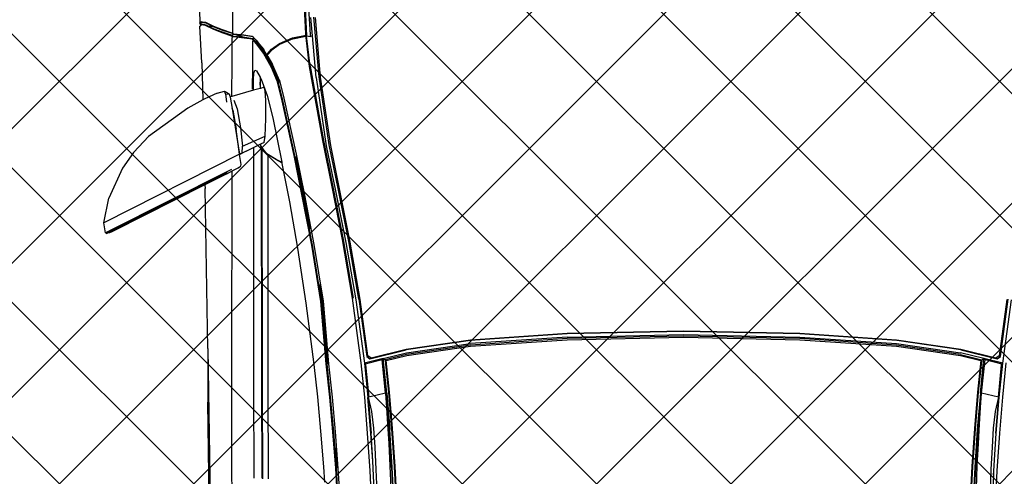
# Model space of a CAD drawing. Units: inches. Extents: x 2167 to 2589, y 1680 to 2489.
# Tile 17 of 38: x 2335 to 2387, y 1772 to 1796. Entities that reach past the tile are written whole.
import ezdxf

# ---------------------------------------------------------------- set-up
doc = ezdxf.new("R2010")
doc.units = ezdxf.units.IN
doc.header["$MEASUREMENT"] = 0
doc.layers.get('0').update_dxf_attribs({"color": 250})
doc.layers.add('C-PRKG-VEHS', color=8, linetype='Continuous', lineweight=13)
doc.layers.add('L-PVMT-PATT', color=252, linetype='Continuous', lineweight=13)
doc.layers.add('Edges', color=250, linetype='Continuous')

# ---------------------------------------------------------------- blocks, each defined once
blk = doc.blocks.new('Nissan Qashqai pl')
at = {"layer": 'Edges'}
for p, q in [((9.2789, 12.5131), (9.1617, 12.5292)), ((9.2669, 12.5088), (9.1605, 12.5233)), ((9.1612, 12.5208), (9.2656, 12.5065)), ((9.2656, 12.5065), (9.2669, 12.5088)), ((9.2707, 12.5028), (9.2669, 12.5088)), ((9.2789, 12.5131), (9.2704, 12.4783)), ((9.2724, 12.4804), (9.2799, 12.5114)), ((9.2783, 12.5191), (9.3422, 12.5126)), ((9.2799, 12.5114), (9.2789, 12.5131)), ((9.3427, 12.5066), (9.2789, 12.5131)), ((9.2819, 12.5112), (9.2799, 12.5114)), ((9.2803, 12.5116), (9.2822, 12.5118)), ((9.3418, 12.5051), (9.2819, 12.5112)), ((9.3422, 12.5126), (9.4088, 12.507)), ((9.2694, 12.5006), (9.2535, 12.4354)), ((9.2543, 12.4356), (9.2707, 12.5028)), ((9.2656, 12.5065), (9.2694, 12.5006)), ((9.2707, 12.5028), (9.2694, 12.5006)), ((9.3418, 12.5051), (9.3346, 12.4741)), ((9.342, 12.5059), (9.3418, 12.5051)), ((9.3687, 12.5), (9.342, 12.5059)), ((9.4087, 12.5003), (9.342, 12.5059)), ((9.4093, 12.5011), (9.3427, 12.5066)), ((9.3992, 12.496), (9.3687, 12.5)), ((9.4347, 12.494), (9.3992, 12.496)), ((9.4087, 12.5003), (9.4688, 12.4968)), ((9.4088, 12.507), (9.4782, 12.5024)), ((9.4785, 12.4965), (9.4093, 12.5011)), ((9.4761, 12.4919), (9.4347, 12.494)), ((9.4688, 12.4968), (9.4789, 12.4964)), ((9.5168, 12.4903), (9.4761, 12.4919)), ((9.4782, 12.5024), (9.5503, 12.4987)), ((9.4789, 12.4964), (9.4785, 12.4965)), ((9.4862, 12.4961), (9.4785, 12.4965)), ((9.4789, 12.4964), (9.4862, 12.4961)), ((9.4862, 12.4961), (9.514, 12.4949)), ((9.2704, 12.4783), (9.2598, 12.4348)), ((9.2629, 12.435), (9.2726, 12.4746)), ((9.2649, 12.4348), (9.2741, 12.4725)), ((9.2724, 12.4804), (9.2704, 12.4783)), ((9.2726, 12.4746), (9.2704, 12.4783)), ((9.3346, 12.4718), (9.2704, 12.4783)), ((9.3346, 12.4741), (9.2724, 12.4804)), ((9.2746, 12.4744), (9.2726, 12.4746)), ((9.2741, 12.4725), (9.3326, 12.4666)), ((9.333, 12.4685), (9.2746, 12.4744)), ((9.3346, 12.4741), (9.3344, 12.4733)), ((9.3344, 12.4733), (9.4017, 12.4677)), ((9.3344, 12.4733), (9.3611, 12.4715)), ((9.3346, 12.4718), (9.4018, 12.4661)), ((9.3326, 12.4666), (9.4, 12.4609)), ((9.4004, 12.4629), (9.333, 12.4685)), ((9.3611, 12.4715), (9.3918, 12.4695)), ((9.3918, 12.4695), (9.4276, 12.4674)), ((9.4, 12.4609), (9.4706, 12.4561)), ((9.4709, 12.4581), (9.4004, 12.4629)), ((9.4017, 12.4677), (9.472, 12.463)), ((9.4018, 12.4661), (9.472, 12.4614)), ((9.4276, 12.4674), (9.4694, 12.4654)), ((9.4694, 12.4654), (9.5105, 12.4637)), ((9.4706, 12.4561), (9.5443, 12.4522)), ((9.5446, 12.4542), (9.4709, 12.4581)), ((9.472, 12.463), (9.5454, 12.4591)), ((9.472, 12.4614), (9.5454, 12.4576)), ((9.2535, 12.4354), (9.2362, 12.3167)), ((9.2543, 12.4356), (9.2371, 12.3169)), ((9.2426, 12.3164), (9.2598, 12.4348)), ((9.2629, 12.435), (9.2457, 12.3164)), ((9.2476, 12.3163), (9.2649, 12.4348)), ((9.2362, 12.3167), (9.2241, 12.1376)), ((9.2371, 12.3169), (9.2249, 12.1376)), ((9.2305, 12.1375), (9.2426, 12.3164)), ((9.2457, 12.3164), (9.2335, 12.1374)), ((9.2355, 12.1374), (9.2476, 12.3163)), ((9.2241, 12.1376), (9.2195, 11.9221)), ((9.2249, 12.1376), (9.2203, 11.9221)), ((9.2259, 11.9221), (9.2305, 12.1375)), ((9.2335, 12.1374), (9.2289, 11.9221)), ((9.2308, 11.9221), (9.2355, 12.1374)), ((9.2195, 11.9221), (9.2241, 11.7066)), ((9.2203, 11.9221), (9.2249, 11.7065)), ((9.2305, 11.7067), (9.2259, 11.9221)), ((9.2289, 11.9221), (9.2335, 11.7067)), ((9.2355, 11.7068), (9.2308, 11.9221)), ((9.2241, 11.7066), (9.2362, 11.5274)), ((9.2249, 11.7065), (9.2371, 11.5273)), ((9.2305, 11.7067), (9.2426, 11.5277)), ((9.2335, 11.7067), (9.2457, 11.5277)), ((9.2476, 11.5278), (9.2355, 11.7068)), ((9.2362, 11.5274), (9.2535, 11.4087)), ((9.2371, 11.5273), (9.2543, 11.4085)), ((9.2598, 11.4093), (9.2426, 11.5277)), ((9.2457, 11.5277), (9.2629, 11.4092)), ((9.2649, 11.4094), (9.2476, 11.5278)), ((9.2535, 11.4087), (9.2694, 11.3436)), ((9.2707, 11.3414), (9.2543, 11.4085)), ((9.2704, 11.3659), (9.2598, 11.4093)), ((9.2629, 11.4092), (9.2726, 11.3695)), ((9.2741, 11.3716), (9.2649, 11.4094)), ((9.4, 11.3832), (9.3326, 11.3776)), ((9.333, 11.3757), (9.4004, 11.3813)), ((9.3346, 11.3724), (9.4018, 11.378)), ((9.4706, 11.388), (9.4, 11.3832)), ((9.4004, 11.3813), (9.4709, 11.3861)), ((9.472, 11.3812), (9.4017, 11.3765)), ((9.472, 11.3828), (9.4018, 11.378)), ((9.4694, 11.3788), (9.4276, 11.3767)), ((9.5105, 11.3805), (9.4694, 11.3788)), ((9.5443, 11.3919), (9.4706, 11.388)), ((9.4709, 11.3861), (9.5446, 11.39)), ((9.5454, 11.3866), (9.472, 11.3828)), ((9.472, 11.3812), (9.5454, 11.3851)), ((9.3346, 11.3724), (9.2704, 11.3659)), ((9.2704, 11.3659), (9.2726, 11.3695)), ((9.2704, 11.3659), (9.2724, 11.3637)), ((9.2704, 11.3659), (9.2789, 11.331)), ((9.3346, 11.37), (9.2724, 11.3637)), ((9.2799, 11.3328), (9.2724, 11.3637)), ((9.2726, 11.3695), (9.2746, 11.3697)), ((9.3326, 11.3776), (9.2741, 11.3716)), ((9.2746, 11.3697), (9.333, 11.3757)), ((9.4017, 11.3765), (9.3344, 11.3708)), ((9.3611, 11.3727), (9.3344, 11.3708)), ((9.3344, 11.3708), (9.3346, 11.37)), ((9.3346, 11.37), (9.3418, 11.3391)), ((9.3918, 11.3747), (9.3611, 11.3727)), ((9.4276, 11.3767), (9.3918, 11.3747)), ((9.2694, 11.3436), (9.2656, 11.3376)), ((9.2669, 11.3354), (9.2707, 11.3414)), ((9.2694, 11.3436), (9.2707, 11.3414)), ((9.342, 11.3383), (9.3687, 11.3441)), ((9.342, 11.3383), (9.4087, 11.3438)), ((9.4093, 11.3431), (9.3427, 11.3375)), ((9.3687, 11.3441), (9.3992, 11.3482)), ((9.3992, 11.3482), (9.4347, 11.3502)), ((9.4605, 11.3465), (9.4087, 11.3438)), ((9.4782, 11.3418), (9.4088, 11.3371)), ((9.4605, 11.3465), (9.4093, 11.3431)), ((9.4347, 11.3502), (9.4761, 11.3522)), ((9.514, 11.3492), (9.4605, 11.3465)), ((9.4761, 11.3522), (9.5168, 11.3539)), ((9.5503, 11.3455), (9.4782, 11.3418)), ((9.1612, 11.3233), (9.0546, 11.3048)), ((9.2783, 11.3251), (9.1584, 11.3091)), ((9.1605, 11.3208), (9.2669, 11.3354)), ((9.2656, 11.3376), (9.1612, 11.3233)), ((9.1617, 11.315), (9.2789, 11.331)), ((9.2669, 11.3354), (9.2656, 11.3376)), ((9.3422, 11.3316), (9.2783, 11.3251)), ((9.2789, 11.331), (9.3427, 11.3375)), ((9.2789, 11.331), (9.2799, 11.3327)), ((9.2799, 11.3328), (9.2819, 11.333)), ((9.2799, 11.3327), (9.2799, 11.3328)), ((9.2799, 11.3327), (9.2811, 11.3325)), ((9.2819, 11.333), (9.3418, 11.3391)), ((9.3418, 11.3391), (9.342, 11.3383)), ((9.4088, 11.3371), (9.3422, 11.3316)), ((9.0546, 11.3048), (8.9591, 11.2859)), ((9.1584, 11.3091), (9.0495, 11.2906)), ((9.0497, 11.2918), (9.1586, 11.3104)), ((9.1605, 11.3208), (9.0538, 11.3023)), ((9.0552, 11.2965), (9.1617, 11.315)), ((9.0495, 11.2906), (8.9521, 11.2715)), ((8.9522, 11.2728), (9.0497, 11.2918)), ((9.0538, 11.3023), (8.9583, 11.2833)), ((8.9598, 11.2775), (9.0552, 11.2965)), ((8.8754, 11.2687), (8.7491, 11.2501)), ((8.8666, 11.2554), (8.9522, 11.2728)), ((8.9521, 11.2715), (8.8666, 11.2541)), ((8.9583, 11.2833), (8.8745, 11.266)), ((8.9591, 11.2859), (8.8754, 11.2687)), ((8.8761, 11.2602), (8.9598, 11.2775)), ((9.2801, 11.2648), (9.3418, 11.2713)), ((9.3419, 11.2685), (9.2804, 11.262)), ((9.3418, 11.2713), (9.4064, 11.277)), ((9.4062, 11.2729), (9.3418, 11.2671)), ((9.4063, 11.2743), (9.3419, 11.2685)), ((9.4735, 11.2779), (9.4062, 11.2729)), ((9.4736, 11.2793), (9.4063, 11.2743)), ((9.4064, 11.277), (9.4739, 11.282)), ((9.4727, 11.2808), (9.4362, 11.278)), ((9.4727, 11.2808), (9.4732, 11.2808)), ((9.5437, 11.2822), (9.4735, 11.2779)), ((9.5438, 11.2836), (9.4736, 11.2793)), ((9.4739, 11.282), (9.5443, 11.2863)), ((8.7491, 11.2501), (8.6386, 11.2404)), ((8.7287, 11.2307), (8.8666, 11.2554)), ((8.8666, 11.2541), (8.7292, 11.2295)), ((8.8745, 11.266), (8.7481, 11.2473)), ((8.7496, 11.2416), (8.8761, 11.2602)), ((9.0591, 11.2377), (9.1639, 11.2546)), ((9.1644, 11.2503), (9.06, 11.2335)), ((9.1645, 11.2518), (9.0601, 11.235)), ((9.133, 11.2481), (9.1647, 11.2532)), ((9.1639, 11.2546), (9.2801, 11.2648)), ((9.2803, 11.2606), (9.1644, 11.2503)), ((9.2804, 11.262), (9.1645, 11.2518)), ((9.1647, 11.2532), (9.1668, 11.2533)), ((9.2804, 11.2635), (9.1668, 11.2533)), ((9.3418, 11.2671), (9.2803, 11.2606)), ((9.3416, 11.2442), (9.4048, 11.2501)), ((9.4048, 11.2501), (9.471, 11.2554)), ((9.471, 11.2554), (9.4997, 11.2573)), ((8.7481, 11.2473), (8.6375, 11.2376)), ((8.6721, 11.2348), (8.6387, 11.2319)), ((8.7496, 11.2416), (8.6721, 11.2348)), ((8.6721, 11.2348), (8.6733, 11.2313)), ((9.0601, 11.235), (8.8941, 11.2023)), ((8.9679, 11.2201), (9.0591, 11.2377)), ((9.06, 11.2335), (8.9696, 11.2157)), ((9.1676, 11.2229), (9.2814, 11.2377)), ((9.2814, 11.2377), (9.3416, 11.2442)), ((8.6683, 11.2226), (8.6197, 11.2201)), ((8.6203, 11.2213), (8.6721, 11.2241)), ((8.6699, 11.231), (8.622, 11.228)), ((8.671, 11.2227), (8.6683, 11.2226)), ((8.6721, 11.2312), (8.6699, 11.231)), ((8.6721, 11.2241), (8.671, 11.2227)), ((8.6716, 11.2199), (8.671, 11.2227)), ((8.6759, 11.1982), (8.6716, 11.2199)), ((8.6721, 11.2312), (8.6721, 11.2318)), ((8.6721, 11.2241), (8.6733, 11.2313)), ((8.6733, 11.2313), (8.6721, 11.2312)), ((8.7287, 11.2307), (8.6721, 11.2241)), ((8.6721, 11.2241), (8.6727, 11.2229)), ((8.6772, 11.1988), (8.6721, 11.2241)), ((8.6753, 11.2232), (8.6727, 11.2229)), ((8.6777, 11.1984), (8.6727, 11.2229)), ((8.7292, 11.2295), (8.6753, 11.2232)), ((8.8918, 11.205), (8.9679, 11.2201)), ((8.9696, 11.2157), (8.8942, 11.2009)), ((8.9318, 11.211), (8.9704, 11.2185)), ((8.9704, 11.2185), (8.9708, 11.2185)), ((8.9708, 11.2185), (9.03, 11.2304)), ((9.0656, 11.207), (9.1676, 11.2229)), ((8.6864, 11.1736), (8.6759, 11.1982)), ((8.6875, 11.1744), (8.6772, 11.1988)), ((8.6777, 11.1984), (8.6883, 11.1737)), ((8.7881, 11.1821), (8.8918, 11.205)), ((8.8941, 11.2023), (8.7925, 11.1802)), ((8.8942, 11.2009), (8.7931, 11.1789)), ((8.8961, 11.204), (8.9318, 11.211)), ((8.9797, 11.1924), (9.0656, 11.207)), ((8.7931, 11.1789), (8.7574, 11.1704)), ((8.7575, 11.1744), (8.7881, 11.1821)), ((8.7925, 11.1802), (8.7591, 11.1723)), ((8.8245, 11.1613), (8.9063, 11.1779)), ((8.9021, 11.1697), (8.9063, 11.1779)), ((8.9075, 11.1781), (8.9041, 11.1717)), ((8.9063, 11.1779), (8.9075, 11.1781)), ((8.9075, 11.1781), (8.9087, 11.1783)), ((8.9087, 11.1783), (8.9797, 11.1924)), ((8.697, 11.1592), (8.6864, 11.1736)), ((8.6979, 11.1603), (8.6875, 11.1744)), ((8.6883, 11.1737), (8.6987, 11.1597)), ((8.7055, 11.1514), (8.697, 11.1592)), ((8.6987, 11.1596), (8.6979, 11.1603)), ((8.6987, 11.1597), (8.6988, 11.1596)), ((8.6987, 11.1596), (8.6988, 11.1596)), ((8.6996, 11.1588), (8.6987, 11.1596)), ((8.6988, 11.1596), (8.6996, 11.1588)), ((8.7302, 11.1602), (8.7032, 11.145)), ((8.7312, 11.1591), (8.7042, 11.144)), ((8.7075, 11.1487), (8.7346, 11.1636)), ((8.7108, 11.1523), (8.7257, 11.1609)), ((8.7108, 11.1523), (8.7248, 11.1605)), ((8.7248, 11.1605), (8.7257, 11.1609)), ((8.7508, 11.1722), (8.7257, 11.1609)), ((8.7529, 11.17), (8.7302, 11.1602)), ((8.7574, 11.1704), (8.7312, 11.1591)), ((8.7346, 11.1636), (8.7577, 11.1732)), ((8.7346, 11.1636), (8.7491, 11.1703)), ((8.7491, 11.1703), (8.7576, 11.1743)), ((8.7508, 11.1722), (8.7491, 11.1703)), ((8.7532, 11.1733), (8.7508, 11.1722)), ((8.7529, 11.17), (8.7577, 11.1732)), ((8.757, 11.1718), (8.7529, 11.17)), ((8.7532, 11.1733), (8.7575, 11.1744)), ((8.7587, 11.1722), (8.757, 11.1718)), ((8.7575, 11.1744), (8.7576, 11.1743)), ((8.7576, 11.1743), (8.7582, 11.1734)), ((8.7577, 11.1732), (8.7582, 11.1734)), ((8.7582, 11.1734), (8.759, 11.1725)), ((8.759, 11.1725), (8.7587, 11.1722)), ((8.7591, 11.1723), (8.7587, 11.1722)), ((8.759, 11.1725), (8.7591, 11.1723)), ((8.7828, 11.1508), (8.8245, 11.1613)), ((8.8893, 11.1486), (8.9021, 11.1697)), ((8.9041, 11.1717), (8.8927, 11.1528)), ((8.7042, 11.144), (8.687, 11.131)), ((8.6884, 11.1371), (8.6973, 11.144)), ((8.6917, 11.1371), (8.7075, 11.1487)), ((8.7032, 11.145), (8.6927, 11.1371)), ((8.6973, 11.144), (8.698, 11.1446)), ((8.698, 11.1446), (8.6981, 11.1446)), ((8.7071, 11.15), (8.6981, 11.1446)), ((8.6996, 11.1588), (8.6996, 11.1588)), ((8.7062, 11.1527), (8.6996, 11.1588)), ((8.6996, 11.1588), (8.7062, 11.1527)), ((8.707, 11.15), (8.7055, 11.1514)), ((8.7067, 11.1522), (8.7062, 11.1527)), ((8.7083, 11.1508), (8.7067, 11.1522)), ((8.707, 11.15), (8.7083, 11.1508)), ((8.7071, 11.15), (8.707, 11.15)), ((8.707, 11.15), (8.707, 11.15)), ((8.7083, 11.1508), (8.7071, 11.15)), ((8.7083, 11.1507), (8.7102, 11.1519)), ((8.7083, 11.1508), (8.7083, 11.1507)), ((8.7102, 11.1519), (8.7108, 11.1523)), ((8.7524, 11.1401), (8.7828, 11.1508)), ((8.7748, 11.1475), (8.7678, 11.1453)), ((8.7678, 11.1453), (8.7698, 11.1385)), ((8.7916, 11.1488), (8.7748, 11.1475)), ((8.8259, 11.1483), (8.7916, 11.1488)), ((8.8585, 11.1473), (8.8259, 11.1483)), ((8.87, 11.1455), (8.8585, 11.1473)), ((8.8771, 11.1054), (8.8585, 11.1473)), ((8.87, 11.1455), (8.8734, 11.1385)), ((8.8893, 11.1486), (8.8751, 11.1387)), ((8.879, 11.1402), (8.881, 11.1418)), ((8.881, 11.1418), (8.8893, 11.1486)), ((9.3225, 11.1421), (8.881, 11.1418)), ((8.8913, 11.1506), (8.8893, 11.1486)), ((8.8927, 11.1528), (8.8913, 11.1506)), ((9.3225, 11.1531), (8.8927, 11.1528)), ((9.3198, 11.1403), (9.4922, 11.1409)), ((9.4936, 11.1538), (9.3225, 11.1531)), ((9.4936, 11.1428), (9.3225, 11.1421)), ((8.6703, 11.1081), (8.6727, 11.1235)), ((8.6714, 11.1088), (8.6737, 11.1245)), ((8.6727, 11.1235), (8.6737, 11.1245)), ((8.6737, 11.1245), (8.6746, 11.1253)), ((8.6805, 11.1309), (8.6746, 11.1253)), ((8.6746, 11.1253), (8.6785, 11.1253)), ((8.6777, 11.1246), (8.6755, 11.1099)), ((8.6788, 11.1237), (8.6764, 11.1083)), ((8.6785, 11.1253), (8.6777, 11.1246)), ((8.6815, 11.128), (8.6785, 11.1253)), ((8.687, 11.131), (8.6788, 11.1237)), ((8.6805, 11.1309), (8.6884, 11.1371)), ((8.6815, 11.128), (8.6818, 11.1288)), ((8.6817, 11.1282), (8.6815, 11.128)), ((8.6859, 11.132), (8.6817, 11.1282)), ((8.6817, 11.1282), (8.6818, 11.1288)), ((8.6818, 11.1288), (8.6902, 11.136)), ((8.6818, 11.1238), (8.7026, 11.1238)), ((8.6927, 11.1371), (8.6859, 11.132)), ((8.6884, 11.1371), (8.6917, 11.1371)), ((8.6902, 11.136), (8.6917, 11.1371)), ((8.6923, 11.1371), (8.6927, 11.1371)), ((8.7026, 11.1238), (8.7026, 11.1239)), ((8.7026, 11.1238), (8.7072, 11.1239)), ((8.7072, 11.1239), (8.7072, 11.1239)), ((8.7072, 11.1239), (8.7273, 11.1239)), ((8.7273, 11.1239), (8.7273, 11.124)), ((8.7273, 11.1239), (8.7354, 11.124)), ((8.7354, 11.1241), (8.7354, 11.124)), ((8.7354, 11.124), (8.742, 11.124)), ((8.7361, 11.1283), (8.7373, 11.1314)), ((8.7415, 11.1265), (8.7361, 11.1283)), ((8.7373, 11.1314), (8.7492, 11.1383)), ((8.7534, 11.1257), (8.7415, 11.1265)), ((8.742, 11.1241), (8.742, 11.124)), ((8.742, 11.124), (8.742, 11.1241)), ((8.742, 11.124), (8.742, 11.124)), ((8.742, 11.124), (8.7426, 11.124)), ((8.7426, 11.1241), (8.7426, 11.124)), ((8.7426, 11.124), (8.7433, 11.124)), ((8.7433, 11.1241), (8.7433, 11.124)), ((8.7433, 11.124), (8.7711, 11.1241)), ((8.7492, 11.1383), (8.7524, 11.1401)), ((8.7492, 11.1383), (8.7572, 11.1379)), ((8.7711, 11.1241), (8.7516, 11.1241)), ((8.7718, 11.126), (8.7534, 11.1257)), ((8.7572, 11.1379), (8.7698, 11.1383)), ((8.7698, 11.1385), (8.7583, 11.1382)), ((8.7698, 11.1385), (8.7698, 11.1383)), ((8.7698, 11.1383), (8.7733, 11.126)), ((8.7733, 11.126), (8.7718, 11.126)), ((8.7733, 11.126), (8.7849, 11.0859)), ((8.8734, 11.1385), (8.8793, 11.1261)), ((8.8734, 11.1385), (8.8768, 11.1385)), ((8.8751, 11.1387), (8.8768, 11.1385)), ((8.8768, 11.1385), (8.879, 11.1402)), ((8.879, 11.1402), (9.3198, 11.1403)), ((9.3194, 11.1262), (8.8793, 11.1261)), ((8.8793, 11.1261), (8.8815, 11.1214)), ((9.4919, 11.1269), (9.3194, 11.1262)), ((8.6684, 11.0892), (8.6703, 11.1081)), ((8.6697, 11.0922), (8.6714, 11.1088)), ((8.6698, 11.0925), (8.6755, 11.1099)), ((8.6754, 11.1089), (8.6735, 11.0898)), ((8.6764, 11.1082), (8.6744, 11.0891)), ((8.6755, 11.1099), (8.6754, 11.1089)), ((8.6764, 11.1082), (8.6764, 11.1083)), ((8.8429, 11.1016), (8.8771, 11.1054)), ((8.8895, 11.1048), (8.8771, 11.1054)), ((8.8815, 11.1214), (8.892, 11.0998)), ((8.8815, 11.1214), (8.8895, 11.1048)), ((8.8908, 11.1021), (8.8895, 11.1048)), ((8.8906, 11.1024), (8.8895, 11.1048)), ((8.5326, 11.0874), (8.6675, 11.0866)), ((8.6616, 11.0683), (8.6675, 11.0862)), ((8.6718, 11.0868), (8.6657, 11.0684)), ((8.6667, 11.0857), (8.6675, 11.0862)), ((8.6674, 11.0864), (8.6675, 11.0865)), ((8.6675, 11.0865), (8.6675, 11.0866)), ((8.6676, 11.0866), (8.6675, 11.0866)), ((8.6675, 11.0862), (8.6679, 11.0864)), ((8.6676, 11.0864), (8.6677, 11.0866)), ((8.6677, 11.0866), (8.6676, 11.0866)), ((8.6682, 11.0866), (8.6677, 11.0866)), ((8.6679, 11.0864), (8.6682, 11.0866)), ((8.6682, 11.087), (8.6684, 11.0888)), ((8.6692, 11.0876), (8.6682, 11.0866)), ((8.6682, 11.087), (8.6692, 11.0876)), ((8.6682, 11.0866), (8.6682, 11.087)), ((8.6684, 11.0888), (8.6684, 11.0892)), ((8.6684, 11.0888), (8.6685, 11.089)), ((8.6692, 11.0876), (8.6697, 11.0922)), ((8.6697, 11.0922), (8.6698, 11.0925)), ((8.6729, 11.0874), (8.6718, 11.0868)), ((8.674, 11.0864), (8.6728, 11.0858)), ((8.6733, 11.0875), (8.6729, 11.0874)), ((8.6735, 11.0898), (8.6733, 11.0875)), ((8.6742, 11.0866), (8.674, 11.0864)), ((8.6744, 11.0891), (8.6742, 11.0866)), ((8.6744, 11.0866), (8.6742, 11.0866)), ((8.6744, 11.0864), (8.6744, 11.0866)), ((8.6773, 11.0865), (8.6744, 11.0866)), ((8.6791, 11.0864), (8.677, 11.0864)), ((8.6791, 11.0865), (8.6773, 11.0865)), ((8.6791, 11.0865), (8.6791, 11.0864)), ((8.6878, 11.0864), (8.6791, 11.0865)), ((8.7205, 11.0863), (8.6791, 11.0864)), ((8.6878, 11.0864), (8.6791, 11.0864)), ((8.6878, 11.0865), (8.6878, 11.0864)), ((8.6911, 11.0864), (8.6878, 11.0864)), ((8.7205, 11.0863), (8.6911, 11.0864)), ((8.7849, 11.0859), (8.7205, 11.0863)), ((8.7858, 11.0828), (8.807, 11.0862)), ((8.7917, 11.0895), (8.8075, 11.0955)), ((8.807, 11.0862), (8.8918, 11.0997)), ((8.8102, 11.0874), (8.807, 11.0862)), ((8.8075, 11.0955), (8.8429, 11.1016)), ((8.8102, 11.0874), (8.8455, 11.0936)), ((8.8918, 11.0997), (8.8455, 11.0936)), ((8.8906, 11.1024), (8.8911, 11.1013)), ((8.892, 11.0998), (8.8908, 11.1021)), ((8.8911, 11.1013), (8.8919, 11.0997)), ((8.8911, 11.1013), (8.8919, 11.0998)), ((8.8919, 11.0997), (8.8911, 11.1013)), ((8.8919, 11.0997), (8.8918, 11.0997)), ((8.8918, 11.0997), (9.0186, 10.8486)), ((8.892, 11.0998), (8.8919, 11.0998)), ((8.8919, 11.0998), (8.8919, 11.0997)), ((8.8919, 11.0997), (8.8919, 11.0997)), ((8.9106, 11.1029), (8.892, 11.0998)), ((8.892, 11.0998), (8.892, 11.0998)), ((8.9131, 11.102), (8.9106, 11.1029)), ((8.9171, 11.0978), (8.9131, 11.102)), ((8.9171, 11.0978), (8.917, 11.0974)), ((8.9171, 11.0978), (8.9233, 11.0855)), ((9.4673, 11.0852), (9.6358, 11.0866)), ((8.6556, 11.0524), (8.6616, 11.0683)), ((8.6657, 11.0684), (8.6598, 11.0529)), ((8.6606, 11.0674), (8.6667, 11.0857)), ((8.6728, 11.0858), (8.6667, 11.0675)), ((8.6742, 11.0858), (8.6743, 11.086)), ((8.7751, 11.0723), (8.7779, 11.0773)), ((8.7798, 11.0739), (8.7751, 11.0723)), ((8.7785, 11.0587), (8.7751, 11.0723)), ((8.7779, 11.0773), (8.7807, 11.0812)), ((8.7798, 11.0739), (8.7807, 11.0812)), ((8.7798, 11.0739), (8.7954, 11.0758)), ((8.7849, 11.0827), (8.7807, 11.0812)), ((8.7849, 11.0859), (8.7856, 11.0834)), ((8.7849, 11.0827), (8.7858, 11.0828)), ((8.7858, 11.0828), (8.7856, 11.0834)), ((8.9232, 11.0779), (8.9194, 11.0854)), ((9.0333, 10.8597), (8.9232, 11.0779)), ((8.9233, 11.0855), (9.2886, 11.0848)), ((8.925, 11.0821), (8.9233, 11.0855)), ((8.928, 11.0762), (8.925, 11.0821)), ((9.0386, 10.8534), (8.9254, 11.0778)), ((8.928, 11.0762), (8.9483, 11.0359)), ((9.2886, 11.0848), (9.4673, 11.0852)), ((8.6472, 11.0366), (8.6546, 11.0516)), ((8.6482, 11.0375), (8.655, 11.0513)), ((8.6608, 11.0521), (8.6534, 11.0369)), ((8.6546, 11.0516), (8.6606, 11.0674)), ((8.6598, 11.0529), (8.655, 11.0432)), ((8.655, 11.0513), (8.6556, 11.0524)), ((8.655, 11.0513), (8.655, 11.0432)), ((8.6667, 11.0675), (8.6608, 11.0521)), ((8.7785, 11.0587), (8.7891, 11.0353)), ((8.646, 11.0289), (8.6468, 11.0337)), ((8.6468, 11.0337), (8.6472, 11.0366)), ((8.647, 11.03), (8.6468, 11.0337)), ((8.647, 11.03), (8.6482, 11.0375)), ((8.6524, 11.0378), (8.651, 11.0302)), ((8.6534, 11.0369), (8.652, 11.0292)), ((8.655, 11.0432), (8.6524, 11.0378)), ((8.7222, 11.0298), (8.7908, 11.0322)), ((8.7891, 11.0353), (8.7908, 11.0322)), ((8.7908, 11.0322), (8.8066, 11.0041)), ((8.9483, 11.0359), (8.9552, 11.0361)), ((8.9483, 11.0359), (9.0343, 10.8656)), ((9.2517, 11.0411), (8.9552, 11.0361)), ((9.2517, 11.0411), (9.5372, 11.0459)), ((9.2517, 11.0411), (9.351, 11.0411)), ((9.641, 11.045), (9.351, 11.0411)), ((8.5838, 11.0251), (8.6489, 11.0263)), ((8.6489, 11.0263), (8.646, 11.0289)), ((8.6498, 11.0273), (8.647, 11.03)), ((8.6527, 11.0286), (8.6489, 11.0263)), ((8.6524, 11.0289), (8.6498, 11.0273)), ((8.651, 11.0302), (8.652, 11.0292)), ((8.652, 11.0292), (8.6524, 11.0289)), ((8.6524, 11.0289), (8.6527, 11.0286)), ((8.6527, 11.0286), (8.6537, 11.0275)), ((8.6547, 11.0265), (8.6537, 11.0275)), ((8.6537, 11.0275), (8.6537, 11.0275)), ((8.7222, 11.0298), (8.6547, 11.0265)), ((8.8066, 11.0041), (8.8591, 10.9315)), ((8.8591, 10.9315), (8.8879, 10.9041)), ((8.8885, 10.9037), (8.8879, 10.9041)), ((8.8885, 10.9037), (8.9173, 10.8831)), ((8.9173, 10.8831), (8.9731, 10.8577)), ((9.0186, 10.8486), (8.9731, 10.8577)), ((9.0374, 10.8517), (9.0186, 10.8486)), ((9.0356, 10.8553), (9.0333, 10.8597)), ((9.0343, 10.8656), (9.0347, 10.8648)), ((9.0347, 10.8648), (9.0362, 10.8619)), ((9.0356, 10.8553), (9.0374, 10.8517)), ((9.0362, 10.8619), (9.037, 10.8603)), ((9.0371, 10.8601), (9.037, 10.8603)), ((9.0371, 10.8601), (9.0376, 10.8591)), ((9.0376, 10.8591), (9.0371, 10.8595)), ((9.0386, 10.8534), (9.0374, 10.8517)), ((9.0376, 10.8591), (9.0386, 10.8534))]:
    blk.add_line(p, q, dxfattribs=at)
blk = doc.blocks.new('car')
blk.add_blockref('Nissan Qashqai pl', (-9.7433, -11.9151))
blk = doc.blocks.new('carr')
blk.add_blockref('car', (0.5124, -0.007))

msp = doc.modelspace()

# ---------------------------------------------------------------- hatches: boundary and pattern name
at = {"layer": 'L-PVMT-PATT'}
h = msp.add_hatch(dxfattribs=at)
h.set_pattern_fill('ANSI37', color=256, scale=40)
h.paths.add_polyline_path([(2417.548, 1783.695), (2417.548, 1846.042), (2239.361, 1846.042), (2239.361, 1687.695), (2369.843, 1687.695), (2369.843, 1696.695), (2375.607, 1696.695), (2416.107, 1696.695), (2417.548, 1696.695)])

# ---------------------------------------------------------------- block references
at = {"layer": 'C-PRKG-VEHS', "xscale": 28.42784210623918, "yscale": 28.42784210623918, "zscale": 28.42784210623918, "rotation": 270}
msp.add_blockref('carr', (2369.852, 1779.037), dxfattribs=at)

doc.saveas('drawing.dxf')
